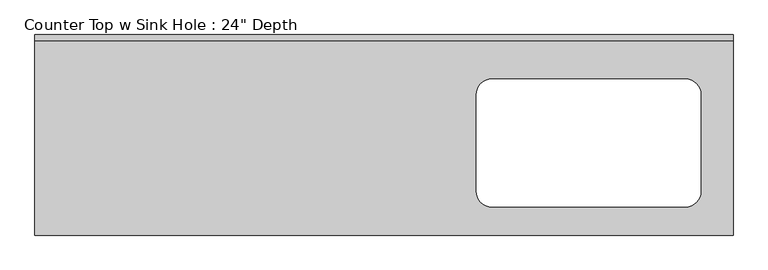
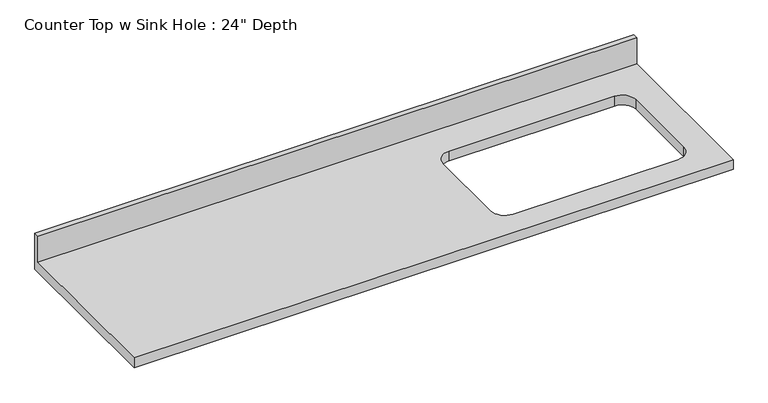
"""IFC4 building model written with IfcOpenShell, lengths in millimetres: furniture geometry."""

from ifc_helpers import new_model, si_unit, frame, origin, place, context, project, spatial, polyline, circle_curve, source, transform, mapped, element, save
from ifc_brep_helpers import plane_surface, revolved_surface, advanced_brep


def furniture_e7d75d8c(model_context):
    return source(origin(), model_context, "Body", "AdvancedBrep", [
        advanced_brep(
        [(-1200.4622951, -635.0, 914.4), (1009.3377049, -635.0, 914.4), (1009.3377049, -19.05, 914.4), (-1200.4622951, -19.05, 914.4), (247.3377049, -139.7, 914.4), (856.9377049, -139.7, 914.4), (907.7377049, -190.5, 914.4), (907.7377049, -495.3, 914.4), (856.9377049, -546.1, 914.4), (247.3377049, -546.1, 914.4), (196.5377049, -495.3, 914.4), (196.5377049, -190.5, 914.4), (1009.3377049, 0.0, 876.3), (1009.3377049, -635.0, 876.3), (-1200.4622951, -635.0, 876.3), (-1200.4622951, 0.0, 876.3), (856.9377049, -139.7, 876.3), (247.3377049, -139.7, 876.3), (196.5377049, -190.5, 876.3), (196.5377049, -495.3, 876.3), (247.3377049, -546.1, 876.3), (856.9377049, -546.1, 876.3), (907.7377049, -495.3, 876.3), (907.7377049, -190.5, 876.3), (-1200.4622951, 0.0, 1016.0), (1009.3377049, 0.0, 1016.0), (-1200.4622951, -19.05, 1016.0), (1009.3377049, -19.05, 1016.0)],
        [
            (0, 1),
            (1, 2),
            (2, 3),
            (3, 0),
            (4, 5),
            (5, 6, circle_curve(frame((856.9377049, -190.5, 914.4), z_axis=(0.0, 0.0, -1.0), x_axis=(1.0, 0.0, 0.0)), 50.8)),
            (6, 7),
            (7, 8, circle_curve(frame((856.9377049, -495.3, 914.4), z_axis=(0.0, 0.0, -1.0), x_axis=(1.0, 0.0, 0.0)), 50.8)),
            (8, 9),
            (9, 10, circle_curve(frame((247.3377049, -495.3, 914.4), z_axis=(0.0, 0.0, -1.0), x_axis=(1.0, 0.0, 0.0)), 50.8)),
            (10, 11),
            (11, 4, circle_curve(frame((247.3377049, -190.5, 914.4), z_axis=(0.0, 0.0, -1.0), x_axis=(1.0, 0.0, 0.0)), 50.8)),
            (12, 13),
            (13, 14),
            (14, 15),
            (15, 12),
            (16, 17),
            (17, 18, circle_curve(frame((247.3377049, -190.5, 876.3), z_axis=(0.0, 0.0, 1.0), x_axis=(1.0, 0.0, 0.0)), 50.8)),
            (18, 19),
            (19, 20, circle_curve(frame((247.3377049, -495.3, 876.3), z_axis=(0.0, 0.0, 1.0), x_axis=(1.0, 0.0, 0.0)), 50.8)),
            (20, 21),
            (21, 22, circle_curve(frame((856.9377049, -495.3, 876.3), z_axis=(0.0, 0.0, 1.0), x_axis=(1.0, 0.0, 0.0)), 50.8)),
            (22, 23),
            (23, 16, circle_curve(frame((856.9377049, -190.5, 876.3), z_axis=(0.0, 0.0, 1.0), x_axis=(1.0, 0.0, 0.0)), 50.8)),
            (15, 24),
            (24, 25),
            (25, 12),
            (14, 0),
            (3, 26),
            (26, 24),
            (13, 1),
            (25, 27),
            (27, 2),
            (26, 27),
            (4, 17),
            (16, 5),
            (11, 18),
            (10, 19),
            (9, 20),
            (8, 21),
            (7, 22),
            (6, 23),
        ],
        [
            plane_surface(frame((-1200.4622951, 0.0, 914.4), z_axis=(0.0, 0.0, 1.0), x_axis=(-1.0, 0.0, 0.0))),
            plane_surface(frame((-1200.4622951, 0.0, 876.3), z_axis=(0.0, 0.0, -1.0), x_axis=(1.0, 0.0, 0.0))),
            plane_surface(frame((1009.3377049, 0.0, 914.4), z_axis=(0.0, 1.0, 0.0), x_axis=(0.0, 0.0, -1.0))),
            plane_surface(frame((-1200.4622951, 0.0, 914.4), z_axis=(-1.0, 0.0, 0.0), x_axis=(0.0, 0.0, -1.0))),
            plane_surface(frame((-1200.4622951, -635.0, 914.4), z_axis=(0.0, -1.0, 0.0), x_axis=(0.0, 0.0, -1.0))),
            plane_surface(frame((1009.3377049, -635.0, 914.4), z_axis=(1.0, 0.0, 0.0), x_axis=(0.0, 0.0, -1.0))),
            plane_surface(frame((-1200.4622951, 0.0, 1016.0), z_axis=(0.0, 0.0, 1.0), x_axis=(0.0, -1.0, 0.0))),
            plane_surface(frame((-1200.4622951, -19.05, 1016.0), z_axis=(0.0, -1.0, 0.0), x_axis=(0.0, 0.0, -1.0))),
            plane_surface(frame((856.9377049, -139.7, 914.4), z_axis=(0.0, -1.0, 0.0), x_axis=(0.0, 0.0, -1.0))),
            revolved_surface(polyline([(298.1377049, -190.5, 914.4), (298.1377049, -190.5, 876.3)]), (247.3377049, -190.5, 876.3), (0.0, 0.0, 1.0)),
            plane_surface(frame((196.5377049, -190.5, 914.4), z_axis=(1.0, 0.0, 0.0), x_axis=(0.0, 0.0, -1.0))),
            revolved_surface(polyline([(298.1377049, -495.3, 914.4), (298.1377049, -495.3, 876.3)]), (247.3377049, -495.3, 876.3), (0.0, 0.0, 1.0)),
            plane_surface(frame((247.3377049, -546.1, 914.4), z_axis=(0.0, 1.0, 0.0), x_axis=(0.0, 0.0, -1.0))),
            revolved_surface(polyline([(907.7377048999999, -495.3, 914.4), (907.7377048999999, -495.3, 876.3)]), (856.9377049, -495.3, 876.3), (0.0, 0.0, 1.0)),
            plane_surface(frame((907.7377049, -495.3, 914.4), z_axis=(-1.0, 0.0, 0.0), x_axis=(0.0, 0.0, -1.0))),
            revolved_surface(polyline([(907.7377048999999, -190.5, 914.4), (907.7377048999999, -190.5, 876.3)]), (856.9377049, -190.5, 876.3), (0.0, 0.0, 1.0)),
        ],
        [
            (0, [[1, 2, 3, 4], [5, 6, 7, 8, 9, 10, 11, 12]]),
            (1, [[13, 14, 15, 16], [17, 18, 19, 20, 21, 22, 23, 24]]),
            (2, [[-16, 25, 26, 27]]),
            (3, [[-15, 28, -4, 29, 30, -25]]),
            (4, [[-1, -28, -14, 31]]),
            (5, [[-13, -27, 32, 33, -2, -31]]),
            (6, [[-30, 34, -32, -26]]),
            (7, [[-34, -29, -3, -33]]),
            (8, [[35, -17, 36, -5]]),
            (9, [[-35, -12, 37, -18]]),
            (10, [[-37, -11, 38, -19]]),
            (11, [[-38, -10, 39, -20]]),
            (12, [[-39, -9, 40, -21]]),
            (13, [[-40, -8, 41, -22]]),
            (14, [[-41, -7, 42, -23]]),
            (15, [[-36, -24, -42, -6]]),
        ],
    ),
    ])


if __name__ == "__main__":
    model = new_model("IFC4")
    model_context = context("Model", 3, world=origin())
    ifc_project = project(units=[si_unit("LENGTHUNIT", "METRE", prefix="MILLI")], contexts=[model_context])
    site = spatial("IfcSite", under=ifc_project)
    building = spatial("IfcBuilding", under=site)
    placement = place(None, origin())
    furniture_shape = furniture_e7d75d8c(model_context)
    element("IfcFurniture", 1, ObjectType="Counter Top w Sink Hole : 24\" Depth", at=placement, inside=building, context=model_context, shape_type="MappedRepresentation", body=[
        mapped(furniture_shape, transform((0.0, 0.0, 0.0), x_axis=(1.0, 0.0, 0.0), y_axis=(0.0, 1.0, 0.0), z_axis=(0.0, 0.0, 1.0))),
    ])
    save(model, "model.ifc")

# Revit data of these elements
# Type "Counter Top w Sink Hole : 24\" Depth"
#   Assembly Code = "C1030400"
#   Counter Thickness = 0' - 1 1/2"
#   Depth = 2' - 1"
#   Height = 3' - 0"
#   Length [instance default] = 8' - 0"
#   Sink Location [instance default] = 2' - 0"
#   Sink Location To Wall [instance default] = 0' - 6"
#   Sink Opening Depth [instance default] = 1' - 3"
#   Sink Opening Width [instance default] = 2' - 3"
#   Counter Top Material = none
#   Default Elevation = 0
# Element 1 (IfcFurniture, "Counter Top w Sink Hole : 24\" Depth")
#   Length = 7' - 3"
#   Sink Location = 5' - 9"
#   Materials on its faces: "Counter Top"
# Materials
#   "Counter Top": class "Wood", colour RGB 226 177 128, transparency 0
